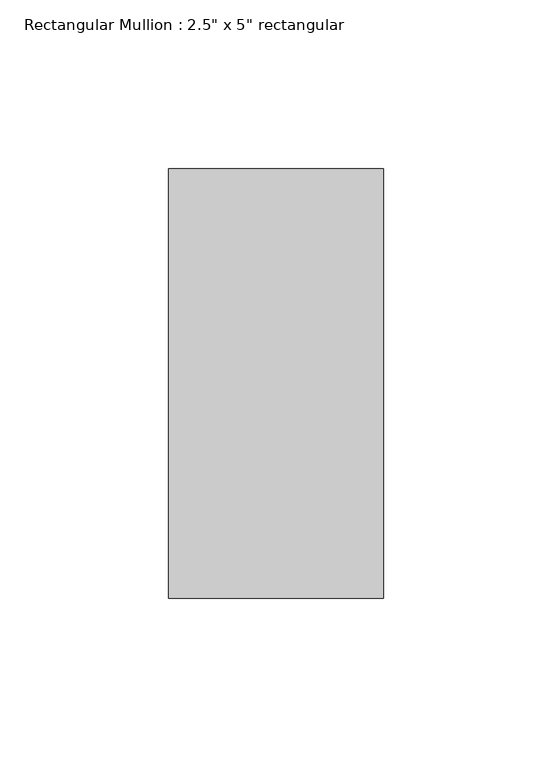
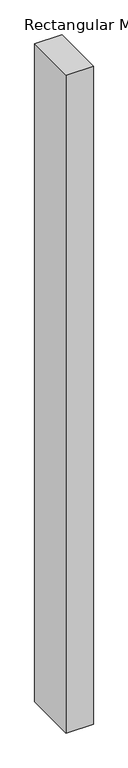
"""IFC4 building model written with IfcOpenShell, lengths in millimetres: member geometry."""

from ifc_helpers import new_model, si_unit, frame, origin, place, context, project, spatial, polyline, outline, extrude, source, transform, mapped, element, save


def member_b7ff1776(model_context):
    return source(origin(), model_context, "Body", "SweptSolid", [
        extrude(outline(polyline([(31.75, 63.5), (31.75, -63.5), (-31.75, -63.5), (-31.75, 63.5), (31.75, 63.5)])), frame((0.0, 0.0, -1624.1102394), z_axis=(0.0, 0.0, 1.0), x_axis=(1.0, 0.0, 0.0)), (0.0, 0.0, 1.0), 1624.1102394),
    ])


if __name__ == "__main__":
    model = new_model("IFC4")
    model_context = context("Model", 3, world=origin())
    ifc_project = project(units=[si_unit("LENGTHUNIT", "METRE", prefix="MILLI")], contexts=[model_context])
    site = spatial("IfcSite", under=ifc_project)
    building = spatial("IfcBuilding", under=site)
    placement = place(None, origin())
    member_shape = member_b7ff1776(model_context)
    element("IfcMember", 1, ObjectType="Rectangular Mullion : 2.5\" x 5\" rectangular", at=placement, inside=building, context=model_context, shape_type="MappedRepresentation", body=[
        mapped(member_shape, transform((0.0, 0.0, 0.0), x_axis=(1.0, 0.0, 0.0), y_axis=(0.0, 1.0, 0.0), z_axis=(0.0, 0.0, 1.0))),
    ])
    save(model, "model.ifc")

# Revit data of these elements
# Type "Rectangular Mullion : 2.5\" x 5\" rectangular"
#   built-in parameter 1007304 = 0.416667 (stored number, unit not read)
#   built-in parameter 1007301 = 0.104167 (stored number, unit not read)
#   built-in parameter 1007300 = 0.104167 (stored number, unit not read)
# Element 1 (IfcMember, "Rectangular Mullion : 2.5\" x 5\" rectangular")
#   Materials on its faces: "Aluminum"
# Materials
#   "Aluminum": class "Metal", colour RGB 247 247 247, transparency 0, Description = "Aluminum 6061", Cost = 0
